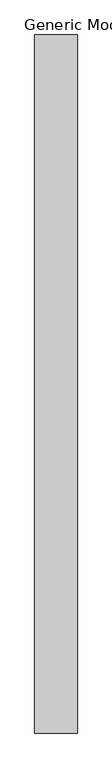
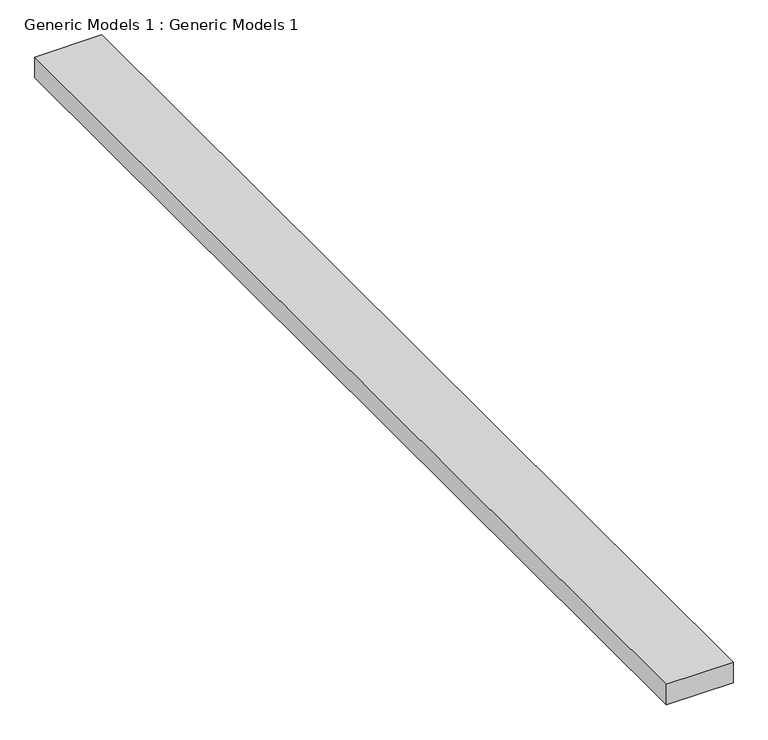
"""IFC4 building model written with IfcOpenShell, lengths in millimetres: proxy geometry, Generic Models 1 : Generic Models 1."""

from ifc_helpers import new_model, si_unit, frame, origin, place, context, project, spatial, polyline, outline, extrude, source, transform, mapped, element, save


def generic_models_1_generic_models_1_103236ad(model_context):
    return source(origin(), model_context, "Body", "SweptSolid", [
        extrude(outline(polyline([(14915.5652909, 554.071634), (14915.5652909, -12687.289536), (14106.5361222, -12687.289536), (14106.5361222, 554.071634), (14915.5652909, 554.071634)])), frame((0.0, 0.0, 18546.8215532), z_axis=(0.0, 0.0, 1.0), x_axis=(1.0, 0.0, 0.0)), (0.0, 0.0, 1.0), 262.6403723),
    ])


if __name__ == "__main__":
    model = new_model("IFC4")
    model_context = context("Model", 3, world=origin())
    ifc_project = project(units=[si_unit("LENGTHUNIT", "METRE", prefix="MILLI")], contexts=[model_context])
    site = spatial("IfcSite", under=ifc_project)
    building = spatial("IfcBuilding", under=site)
    placement = place(None, origin())
    generic_models_1_generic_models_1_shape = generic_models_1_generic_models_1_103236ad(model_context)
    element("IfcBuildingElementProxy", 1, Name="Generic Models 1 : Generic Models 1", ObjectType="Generic Models 1 : Generic Models 1", at=placement, inside=building, context=model_context, shape_type="MappedRepresentation", body=[
        mapped(generic_models_1_generic_models_1_shape, transform((0.0, 0.0, 0.0), x_axis=(1.0, 0.0, 0.0), y_axis=(0.0, 1.0, 0.0), z_axis=(0.0, 0.0, 1.0))),
    ])
    save(model, "model.ifc")
